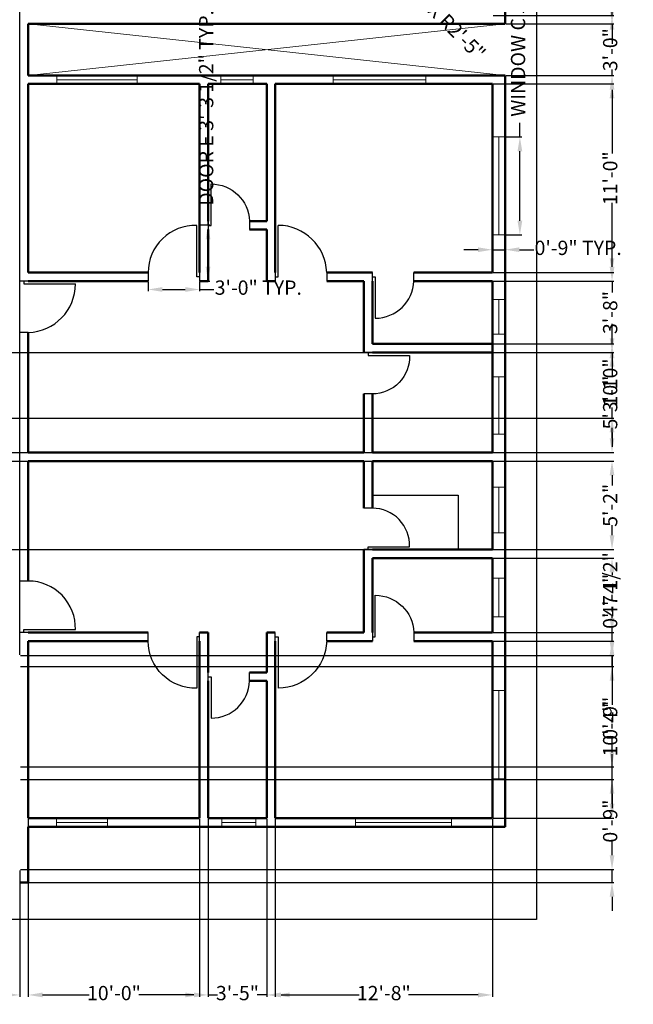
# Model space of a CAD drawing. Units: inches. Extents: x 3237 to 4201, y 2949 to 4053.
# Tile 3 of 5: x 3772 to 4201, y 2949 to 3638. Entities that reach past the tile are written whole.
import ezdxf

# ---------------------------------------------------------------- set-up
doc = ezdxf.new("R2010")
doc.units = ezdxf.units.IN
for name, color, linetype, lineweight in [('A-ANNO-DIMS', 2, 'Continuous', 18), ('A-DOOR', 3, 'Continuous', 25), ('A-FLOR-CASE', 8, 'Continuous', 25), ('A-FLOR-OPEN', 8, 'Continuous', 13), ('A-GLAZ', 4, 'Continuous', 18), ('A-WALL', 7, 'Continuous', 50), ('C-PROP', 6, 'Continuous', 25)]:
    doc.layers.add(name, color=color, linetype=linetype, lineweight=lineweight)
doc.styles.get("Standard").update_dxf_attribs({"font": 'arial.ttf'})
doc.dimstyles.new('ISO-25', dxfattribs={"dimtxt": 10, "dimasz": 10, "dimexe": 1.25, "dimexo": 0.625, "dimtad": 0, "dimdec": 0, "dimlunit": 3, "dimtxsty": 'Standard', "dimcen": 2.5, "dimadec": 0, "dimazin": 0, "dimtfac": 1, "dimtdec": 0, "dimtmove": 0, "dimatfit": 3, "dimfxl": 1, "dimarcsym": 0})

# ---------------------------------------------------------------- blocks, each defined once
blk = doc.blocks.new('DOOR-29-OFFSET-A')
for p, q in [((0, 26), (0, 32)), ((0, 29), (2, 29)), ((2, 29), (2, 0)), ((29, 26), (29, 32))]:
    blk.add_line(p, q)
blk.add_arc((2, 27.02), 27.02, 270, 357.83815)
blk = doc.blocks.new('DOOR-36-OFFSET-A')
for p, q in [((2, 3), (2, 39)), ((0, 6), (0, 0)), ((0, 3), (2, 3)), ((36, 6), (36, 0))]:
    blk.add_line(p, q)
blk.add_arc((2, 4.98), 34.02, 1.71019, 90)
blk = doc.blocks.new('DOOR-29-OFFSET-B')
for p, q in [((27, 3), (27, 32)), ((0, 6), (0, 0)), ((29, 3), (27, 3)), ((29, 6), (29, 0))]:
    blk.add_line(p, q)
blk.add_arc((26.02, 6), 26.02, 87.83815, 180)
blk = doc.blocks.new('DOOR-36-OFFSET-B')
for p, q in [((34, 3), (34, 39)), ((0, 6), (0, 0)), ((36, 3), (34, 3)), ((36, 6), (36, 0))]:
    blk.add_line(p, q)
blk.add_arc((33.01, 6), 33.01, 88.28981, 180)
blk = doc.blocks.new('WIN-61p86IN')
for p, q in [((0, 61.86), (9, 61.86)), ((4.5, 0), (4.5, 61.86)), ((0, 0), (9, 0))]:
    blk.add_line(p, q)
blk = doc.blocks.new('WIN-68p61IN')
for p, q in [((0, 68.61), (9, 68.61)), ((4.5, 0), (4.5, 68.61)), ((0, 0), (9, 0))]:
    blk.add_line(p, q)
blk = doc.blocks.new('COUNTER-L-60x38')
for p, q in [((60, 38), (0, 38)), ((0, 38), (0, 0))]:
    blk.add_line(p, q)
blk = doc.blocks.new('*D23')
at = {"layer": 'A-ANNO-DIMS', "color": 0, "lineweight": -2, "transparency": 16777216}
for p, q in [((3903.41, 3494.25), (3903.41, 3504.25)), ((3898.15, 3494.25), (3904.66, 3494.25)), ((3903.41, 3464.98), (3903.41, 3484.25)), ((3898.15, 3454.98), (3904.66, 3454.98))]:
    blk.add_line(p, q, dxfattribs=at)
at = {"layer": 'A-ANNO-DIMS', "color": 0, "transparency": 16777216}
for points in [[(3901.75, 3484.25), (3905.08, 3484.25), (3903.41, 3494.25)], [(3901.75, 3464.98), (3905.08, 3464.98), (3903.41, 3454.98)]]:
    blk.add_solid(points, dxfattribs=at)
at = {"layer": 'Defpoints', "color": 0, "transparency": 16777216}
for p in [(3897.52, 3494.25), (3903.41, 3494.25), (3897.52, 3454.98)]:
    blk.add_point(p, dxfattribs=at)
at = {"layer": 'A-ANNO-DIMS', "color": 0, "transparency": 16777216, "insert": (3903.41, 3576.25), "char_height": 10, "attachment_point": 5, "rotation": 90}
blk.add_mtext('DOOR E 3\'-3 1/2" TYP.', dxfattribs=at)
blk = doc.blocks.new('*D24')
at = {"layer": 'A-ANNO-DIMS', "color": 0, "lineweight": -2, "transparency": 16777216}
for p, q in [((3861.52, 3454.35), (3861.52, 3447.84)), ((3897.52, 3454.35), (3897.52, 3447.84)), ((3871.52, 3449.09), (3887.52, 3449.09)), ((3897.52, 3449.09), (3907.52, 3449.09))]:
    blk.add_line(p, q, dxfattribs=at)
at = {"layer": 'A-ANNO-DIMS', "color": 0, "transparency": 16777216}
for points in [[(3871.52, 3450.76), (3871.52, 3447.42), (3861.52, 3449.09)], [(3887.52, 3450.76), (3887.52, 3447.42), (3897.52, 3449.09)]]:
    blk.add_solid(points, dxfattribs=at)
at = {"layer": 'Defpoints', "color": 0, "transparency": 16777216}
for p in [(3861.52, 3454.98), (3897.52, 3454.98), (3897.52, 3449.09)]:
    blk.add_point(p, dxfattribs=at)
at = {"layer": 'A-ANNO-DIMS', "color": 0, "transparency": 16777216, "insert": (3938.62, 3449.09), "char_height": 10, "attachment_point": 5}
blk.add_mtext('3\'-0" TYP.', dxfattribs=at)
blk = doc.blocks.new('*D31')
at = {"layer": 'A-ANNO-DIMS', "color": 0, "lineweight": -2, "transparency": 16777216}
for p, q in [((4121.81, 3555.85), (4121.81, 3565.85)), ((4112.15, 3555.85), (4123.06, 3555.85)), ((4121.81, 3497.24), (4121.81, 3545.85)), ((4112.15, 3487.24), (4123.06, 3487.24))]:
    blk.add_line(p, q, dxfattribs=at)
at = {"layer": 'A-ANNO-DIMS', "color": 0, "transparency": 16777216}
for points in [[(4120.15, 3545.85), (4123.48, 3545.85), (4121.81, 3555.85)], [(4120.15, 3497.24), (4123.48, 3497.24), (4121.81, 3487.24)]]:
    blk.add_solid(points, dxfattribs=at)
at = {"layer": 'Defpoints', "color": 0, "transparency": 16777216}
for p in [(4111.52, 3555.85), (4121.81, 3555.85), (4111.52, 3487.24)]:
    blk.add_point(p, dxfattribs=at)
at = {"layer": 'A-ANNO-DIMS', "color": 0, "transparency": 16777216, "insert": (4121.81, 3648.38), "char_height": 10, "attachment_point": 5, "rotation": 90}
blk.add_mtext('WINDOW C 5\'-8 1/2" TYP.', dxfattribs=at)
blk = doc.blocks.new('*D32')
at = {"layer": 'A-ANNO-DIMS', "color": 0, "lineweight": -2, "transparency": 16777216}
for p, q in [((4102.52, 3486.61), (4102.52, 3475.69)), ((4111.52, 3486.61), (4111.52, 3475.69)), ((4092.52, 3476.94), (4082.52, 3476.94)), ((4102.52, 3476.94), (4111.52, 3476.94)), ((4121.52, 3476.94), (4131.52, 3476.94))]:
    blk.add_line(p, q, dxfattribs=at)
at = {"layer": 'A-ANNO-DIMS', "color": 0, "transparency": 16777216}
for points in [[(4092.52, 3478.61), (4092.52, 3475.28), (4102.52, 3476.94)], [(4121.52, 3478.61), (4121.52, 3475.28), (4111.52, 3476.94)]]:
    blk.add_solid(points, dxfattribs=at)
at = {"layer": 'Defpoints', "color": 0, "transparency": 16777216}
for p in [(4102.52, 3487.24), (4111.52, 3487.24), (4111.52, 3476.94)]:
    blk.add_point(p, dxfattribs=at)
at = {"layer": 'A-ANNO-DIMS', "color": 0, "transparency": 16777216, "insert": (4162.62, 3476.94), "char_height": 10, "attachment_point": 5}
blk.add_mtext('0\'-9" TYP.', dxfattribs=at)
blk = doc.blocks.new('*D56')
at = {"layer": 'A-ANNO-DIMS', "color": 0, "lineweight": -2, "transparency": 16777216}
for p, q in [((3777.52, 3078.35), (3777.52, 2953.93)), ((3897.52, 3078.35), (3897.52, 2953.93)), ((3787.52, 2955.18), (3820.19, 2955.18)), ((3887.52, 2955.18), (3854.85, 2955.18))]:
    blk.add_line(p, q, dxfattribs=at)
at = {"layer": 'A-ANNO-DIMS', "color": 0, "transparency": 16777216}
for points in [[(3787.52, 2956.85), (3787.52, 2953.51), (3777.52, 2955.18)], [(3887.52, 2956.85), (3887.52, 2953.51), (3897.52, 2955.18)]]:
    blk.add_solid(points, dxfattribs=at)
at = {"layer": 'Defpoints', "color": 0, "transparency": 16777216}
for p in [(3777.52, 3078.98), (3897.52, 3078.98), (3897.52, 2955.18)]:
    blk.add_point(p, dxfattribs=at)
at = {"layer": 'A-ANNO-DIMS', "color": 0, "transparency": 16777216, "insert": (3837.52, 2955.18), "char_height": 10, "attachment_point": 5}
blk.add_mtext('10\'-0"', dxfattribs=at)
blk = doc.blocks.new('*D57')
at = {"layer": 'A-ANNO-DIMS', "color": 0, "lineweight": -2, "transparency": 16777216}
for p, q in [((3903.52, 3078.35), (3903.52, 2953.93)), ((3944.52, 3078.35), (3944.52, 2953.93)), ((3893.52, 2955.18), (3883.52, 2955.18)), ((3903.52, 2955.18), (3910.11, 2955.18)), ((3944.52, 2955.18), (3937.93, 2955.18)), ((3954.52, 2955.18), (3964.52, 2955.18))]:
    blk.add_line(p, q, dxfattribs=at)
at = {"layer": 'A-ANNO-DIMS', "color": 0, "transparency": 16777216}
for points in [[(3893.52, 2956.85), (3893.52, 2953.51), (3903.52, 2955.18)], [(3954.52, 2956.85), (3954.52, 2953.51), (3944.52, 2955.18)]]:
    blk.add_solid(points, dxfattribs=at)
at = {"layer": 'Defpoints', "color": 0, "transparency": 16777216}
for p in [(3903.52, 3078.98), (3944.52, 3078.98), (3944.52, 2955.18)]:
    blk.add_point(p, dxfattribs=at)
at = {"layer": 'A-ANNO-DIMS', "color": 0, "transparency": 16777216, "insert": (3924.02, 2955.18), "char_height": 10, "attachment_point": 5}
blk.add_mtext('3\'-5"', dxfattribs=at)
blk = doc.blocks.new('*D58')
at = {"layer": 'A-ANNO-DIMS', "color": 0, "lineweight": -2, "transparency": 16777216}
for p, q in [((3950.52, 3078.35), (3950.52, 2953.93)), ((4102.52, 3078.35), (4102.52, 2953.93)), ((3960.52, 2955.18), (4009.19, 2955.18)), ((4092.52, 2955.18), (4043.85, 2955.18))]:
    blk.add_line(p, q, dxfattribs=at)
at = {"layer": 'A-ANNO-DIMS', "color": 0, "transparency": 16777216}
for points in [[(3960.52, 2956.85), (3960.52, 2953.51), (3950.52, 2955.18)], [(4092.52, 2956.85), (4092.52, 2953.51), (4102.52, 2955.18)]]:
    blk.add_solid(points, dxfattribs=at)
at = {"layer": 'Defpoints', "color": 0, "transparency": 16777216}
for p in [(3950.52, 3078.98), (4102.52, 3078.98), (4102.52, 2955.18)]:
    blk.add_point(p, dxfattribs=at)
at = {"layer": 'A-ANNO-DIMS', "color": 0, "transparency": 16777216, "insert": (4026.52, 2955.18), "char_height": 10, "attachment_point": 5}
blk.add_mtext('12\'-8"', dxfattribs=at)
blk = doc.blocks.new('*D61')
at = {"layer": 'A-ANNO-DIMS', "color": 0, "lineweight": -2, "transparency": 16777216}
for p, q in [((3437.15, 3328.98), (4187.57, 3328.98)), ((4186.32, 3318.98), (4186.32, 3311.9)), ((4186.32, 3276.98), (4186.32, 3284.06)), ((3437.15, 3266.98), (4187.57, 3266.98))]:
    blk.add_line(p, q, dxfattribs=at)
at = {"layer": 'A-ANNO-DIMS', "color": 0, "transparency": 16777216}
for points in [[(4184.66, 3318.98), (4187.99, 3318.98), (4186.32, 3328.98)], [(4184.66, 3276.98), (4187.99, 3276.98), (4186.32, 3266.98)]]:
    blk.add_solid(points, dxfattribs=at)
at = {"layer": 'Defpoints', "color": 0, "transparency": 16777216}
for p in [(3436.52, 3328.98), (4186.32, 3328.98), (3436.52, 3266.98)]:
    blk.add_point(p, dxfattribs=at)
at = {"layer": 'A-ANNO-DIMS', "color": 0, "transparency": 16777216, "insert": (4186.32, 3297.98), "char_height": 10, "attachment_point": 5, "rotation": 90}
blk.add_mtext('5\'-2"', dxfattribs=at)
blk = doc.blocks.new('*D62')
at = {"layer": 'A-ANNO-DIMS', "color": 0, "lineweight": -2, "transparency": 16777216}
for p, q in [((3437.15, 3404.98), (4187.57, 3404.98)), ((4186.32, 3394.98), (4186.32, 3387.78)), ((4186.32, 3344.98), (4186.32, 3352.18)), ((3437.15, 3334.98), (4187.57, 3334.98))]:
    blk.add_line(p, q, dxfattribs=at)
at = {"layer": 'A-ANNO-DIMS', "color": 0, "transparency": 16777216}
for points in [[(4184.66, 3394.98), (4187.99, 3394.98), (4186.32, 3404.98)], [(4184.66, 3344.98), (4187.99, 3344.98), (4186.32, 3334.98)]]:
    blk.add_solid(points, dxfattribs=at)
at = {"layer": 'Defpoints', "color": 0, "transparency": 16777216}
for p in [(3436.52, 3404.98), (4186.32, 3404.98), (3436.52, 3334.98)]:
    blk.add_point(p, dxfattribs=at)
at = {"layer": 'A-ANNO-DIMS', "color": 0, "transparency": 16777216, "insert": (4186.32, 3369.98), "char_height": 10, "attachment_point": 5, "rotation": 90}
blk.add_mtext('5\'-10"', dxfattribs=at)
blk = doc.blocks.new('*D63')
at = {"layer": 'A-ANNO-DIMS', "color": 0, "lineweight": -2, "transparency": 16777216}
for p, q in [((4186.32, 3464.98), (4186.32, 3474.98)), ((4103.15, 3454.98), (4187.57, 3454.98)), ((4186.32, 3454.98), (4186.32, 3446.89)), ((4186.32, 3410.98), (4186.32, 3419.07)), ((4103.15, 3410.98), (4187.57, 3410.98)), ((4186.32, 3400.98), (4186.32, 3390.98))]:
    blk.add_line(p, q, dxfattribs=at)
at = {"layer": 'A-ANNO-DIMS', "color": 0, "transparency": 16777216}
for points in [[(4184.66, 3464.98), (4187.99, 3464.98), (4186.32, 3454.98)], [(4184.66, 3400.98), (4187.99, 3400.98), (4186.32, 3410.98)]]:
    blk.add_solid(points, dxfattribs=at)
at = {"layer": 'Defpoints', "color": 0, "transparency": 16777216}
for p in [(4102.52, 3454.98), (4186.32, 3454.98), (4102.52, 3410.98)]:
    blk.add_point(p, dxfattribs=at)
at = {"layer": 'A-ANNO-DIMS', "color": 0, "transparency": 16777216, "insert": (4186.32, 3432.98), "char_height": 10, "attachment_point": 5, "rotation": 90}
blk.add_mtext('3\'-8"', dxfattribs=at)
blk = doc.blocks.new('*D64')
at = {"layer": 'A-ANNO-DIMS', "color": 0, "lineweight": -2, "transparency": 16777216}
for p, q in [((4103.15, 3592.98), (4187.57, 3592.98)), ((4186.32, 3582.98), (4186.32, 3544.31)), ((4186.32, 3470.98), (4186.32, 3509.65)), ((4103.15, 3460.98), (4187.57, 3460.98))]:
    blk.add_line(p, q, dxfattribs=at)
at = {"layer": 'A-ANNO-DIMS', "color": 0, "transparency": 16777216}
for points in [[(4184.66, 3582.98), (4187.99, 3582.98), (4186.32, 3592.98)], [(4184.66, 3470.98), (4187.99, 3470.98), (4186.32, 3460.98)]]:
    blk.add_solid(points, dxfattribs=at)
at = {"layer": 'Defpoints', "color": 0, "transparency": 16777216}
for p in [(4102.52, 3592.98), (4186.32, 3592.98), (4102.52, 3460.98)]:
    blk.add_point(p, dxfattribs=at)
at = {"layer": 'A-ANNO-DIMS', "color": 0, "transparency": 16777216, "insert": (4186.32, 3526.98), "char_height": 10, "attachment_point": 5, "rotation": 90}
blk.add_mtext('11\'-0"', dxfattribs=at)
blk = doc.blocks.new('*D65')
at = {"layer": 'A-ANNO-DIMS', "color": 0, "lineweight": -2, "transparency": 16777216}
for p, q in [((4186.32, 3644.98), (4186.32, 3654.98)), ((4112.15, 3634.98), (4187.57, 3634.98)), ((4186.32, 3634.98), (4186.32, 3630.89)), ((4112.15, 3598.98), (4187.57, 3598.98)), ((4186.32, 3598.98), (4186.32, 3603.07)), ((4186.32, 3588.98), (4186.32, 3578.98))]:
    blk.add_line(p, q, dxfattribs=at)
at = {"layer": 'A-ANNO-DIMS', "color": 0, "transparency": 16777216}
for points in [[(4184.66, 3644.98), (4187.99, 3644.98), (4186.32, 3634.98)], [(4184.66, 3588.98), (4187.99, 3588.98), (4186.32, 3598.98)]]:
    blk.add_solid(points, dxfattribs=at)
at = {"layer": 'Defpoints', "color": 0, "transparency": 16777216}
for p in [(4111.52, 3634.98), (4186.32, 3634.98), (4111.52, 3598.98)]:
    blk.add_point(p, dxfattribs=at)
at = {"layer": 'A-ANNO-DIMS', "color": 0, "transparency": 16777216, "insert": (4186.32, 3616.98), "char_height": 10, "attachment_point": 5, "rotation": 90}
blk.add_mtext('3\'-0"', dxfattribs=at)
blk = doc.blocks.new('*D66')
at = {"layer": 'A-ANNO-DIMS', "color": 0, "lineweight": -2, "transparency": 16777216}
for p, q in [((4186.32, 3698.98), (4186.32, 3708.98)), ((4103.15, 3688.98), (4187.57, 3688.98)), ((4186.32, 3688.98), (4186.32, 3679.1)), ((4186.32, 3640.98), (4186.32, 3650.86)), ((4103.15, 3640.98), (4187.57, 3640.98)), ((4186.32, 3630.98), (4186.32, 3620.98))]:
    blk.add_line(p, q, dxfattribs=at)
at = {"layer": 'A-ANNO-DIMS', "color": 0, "transparency": 16777216}
for points in [[(4184.66, 3698.98), (4187.99, 3698.98), (4186.32, 3688.98)], [(4184.66, 3630.98), (4187.99, 3630.98), (4186.32, 3640.98)]]:
    blk.add_solid(points, dxfattribs=at)
at = {"layer": 'Defpoints', "color": 0, "transparency": 16777216}
for p in [(4102.52, 3688.98), (4186.32, 3688.98), (4102.52, 3640.98)]:
    blk.add_point(p, dxfattribs=at)
at = {"layer": 'A-ANNO-DIMS', "color": 0, "transparency": 16777216, "insert": (4186.32, 3664.98), "char_height": 10, "attachment_point": 5, "rotation": 90}
blk.add_mtext('4\'-0"', dxfattribs=at)
blk = doc.blocks.new('*D70')
at = {"layer": 'A-ANNO-DIMS', "color": 0, "lineweight": -2, "transparency": 16777216}
for p, q in [((4103.15, 3202.98), (4187.57, 3202.98)), ((4186.32, 3192.98), (4186.32, 3158.31)), ((4186.32, 3088.98), (4186.32, 3123.65)), ((4103.15, 3078.98), (4187.57, 3078.98))]:
    blk.add_line(p, q, dxfattribs=at)
at = {"layer": 'A-ANNO-DIMS', "color": 0, "transparency": 16777216}
for points in [[(4184.66, 3192.98), (4187.99, 3192.98), (4186.32, 3202.98)], [(4184.66, 3088.98), (4187.99, 3088.98), (4186.32, 3078.98)]]:
    blk.add_solid(points, dxfattribs=at)
at = {"layer": 'Defpoints', "color": 0, "transparency": 16777216}
for p in [(4102.52, 3202.98), (4186.32, 3202.98), (4102.52, 3078.98)]:
    blk.add_point(p, dxfattribs=at)
at = {"layer": 'A-ANNO-DIMS', "color": 0, "transparency": 16777216, "insert": (4186.32, 3140.98), "char_height": 10, "attachment_point": 5, "rotation": 90}
blk.add_mtext('10\'-4"', dxfattribs=at)
blk = doc.blocks.new('*D71')
at = {"layer": 'A-ANNO-DIMS', "color": 0, "lineweight": -2, "transparency": 16777216}
for p, q in [((4103.15, 3260.98), (4187.57, 3260.98)), ((4186.32, 3250.98), (4186.32, 3249.1)), ((4186.32, 3218.98), (4186.32, 3220.86)), ((4103.15, 3208.98), (4187.57, 3208.98))]:
    blk.add_line(p, q, dxfattribs=at)
at = {"layer": 'A-ANNO-DIMS', "color": 0, "transparency": 16777216}
for points in [[(4184.66, 3250.98), (4187.99, 3250.98), (4186.32, 3260.98)], [(4184.66, 3218.98), (4187.99, 3218.98), (4186.32, 3208.98)]]:
    blk.add_solid(points, dxfattribs=at)
at = {"layer": 'Defpoints', "color": 0, "transparency": 16777216}
for p in [(4102.52, 3260.98), (4186.32, 3260.98), (4102.52, 3208.98)]:
    blk.add_point(p, dxfattribs=at)
at = {"layer": 'A-ANNO-DIMS', "color": 0, "transparency": 16777216, "insert": (4186.32, 3234.98), "char_height": 10, "attachment_point": 5, "rotation": 90}
blk.add_mtext('4\'-4"', dxfattribs=at)
blk = doc.blocks.new('*D74')
at = {"layer": 'A-ANNO-DIMS', "color": 0, "lineweight": -2, "transparency": 16777216}
for p, q in [((4186.32, 3414.98), (4186.32, 3424.98)), ((3377.15, 3404.98), (4187.57, 3404.98)), ((4186.32, 3404.98), (4186.32, 3399.78)), ((4186.32, 3358.98), (4186.32, 3364.18)), ((3377.15, 3358.98), (4187.57, 3358.98)), ((4186.32, 3348.98), (4186.32, 3338.98))]:
    blk.add_line(p, q, dxfattribs=at)
at = {"layer": 'A-ANNO-DIMS', "color": 0, "transparency": 16777216}
for points in [[(4184.66, 3414.98), (4187.99, 3414.98), (4186.32, 3404.98)], [(4184.66, 3348.98), (4187.99, 3348.98), (4186.32, 3358.98)]]:
    blk.add_solid(points, dxfattribs=at)
at = {"layer": 'Defpoints', "color": 0, "transparency": 16777216}
for p in [(3376.52, 3404.98), (4186.32, 3404.98), (3376.52, 3358.98)]:
    blk.add_point(p, dxfattribs=at)
at = {"layer": 'A-ANNO-DIMS', "color": 0, "transparency": 16777216, "insert": (4186.32, 3381.98), "char_height": 10, "attachment_point": 5, "rotation": 90}
blk.add_mtext('3\'-10"', dxfattribs=at)
blk = doc.blocks.new('*D80')
at = {"layer": 'A-ANNO-DIMS', "color": 0, "lineweight": -2, "transparency": 16777216}
for p, q in [((3675.52, 3042.35), (3675.52, 2953.93)), ((3771.52, 3042.35), (3771.52, 2953.93)), ((3685.52, 2955.18), (3709.6, 2955.18)), ((3761.52, 2955.18), (3737.44, 2955.18))]:
    blk.add_line(p, q, dxfattribs=at)
at = {"layer": 'A-ANNO-DIMS', "color": 0, "transparency": 16777216}
for points in [[(3685.52, 2956.85), (3685.52, 2953.51), (3675.52, 2955.18)], [(3761.52, 2956.85), (3761.52, 2953.51), (3771.52, 2955.18)]]:
    blk.add_solid(points, dxfattribs=at)
at = {"layer": 'Defpoints', "color": 0, "transparency": 16777216}
for p in [(3675.52, 3042.98), (3771.52, 3042.98), (3771.52, 2955.18)]:
    blk.add_point(p, dxfattribs=at)
at = {"layer": 'A-ANNO-DIMS', "color": 0, "transparency": 16777216, "insert": (3723.52, 2955.18), "char_height": 10, "attachment_point": 5}
blk.add_mtext('8\'-0"', dxfattribs=at)
blk = doc.blocks.new('*D83')
at = {"layer": 'A-ANNO-DIMS', "color": 0, "lineweight": -2, "transparency": 16777216}
for p, q in [((3713.52, 3960.78), (3703.52, 3960.78)), ((3723.52, 3193.4), (3723.52, 3962.03)), ((3723.52, 3960.78), (3733.4, 3960.78)), ((3771.52, 3960.78), (3761.64, 3960.78)), ((3771.52, 3193.4), (3771.52, 3962.03)), ((3781.52, 3960.78), (3791.52, 3960.78))]:
    blk.add_line(p, q, dxfattribs=at)
at = {"layer": 'A-ANNO-DIMS', "color": 0, "transparency": 16777216}
for points in [[(3713.52, 3962.45), (3713.52, 3959.11), (3723.52, 3960.78)], [(3781.52, 3962.45), (3781.52, 3959.11), (3771.52, 3960.78)]]:
    blk.add_solid(points, dxfattribs=at)
at = {"layer": 'Defpoints', "color": 0, "transparency": 16777216}
for p in [(3771.52, 3960.78), (3723.52, 3192.78), (3771.52, 3192.78)]:
    blk.add_point(p, dxfattribs=at)
at = {"layer": 'A-ANNO-DIMS', "color": 0, "transparency": 16777216, "insert": (3747.52, 3960.78), "char_height": 10, "attachment_point": 5}
blk.add_mtext('4\'-0"', dxfattribs=at)
blk = doc.blocks.new('*D84')
at = {"layer": 'A-ANNO-DIMS', "color": 0, "lineweight": -2, "transparency": 16777216}
for p, q in [((4186.32, 3124.98), (4186.32, 3134.98)), ((3772.15, 3114.98), (4187.57, 3114.98)), ((4186.32, 3105.98), (4186.32, 3114.98)), ((3772.15, 3105.98), (4187.57, 3105.98)), ((4186.32, 3095.98), (4186.32, 3085.98))]:
    blk.add_line(p, q, dxfattribs=at)
at = {"layer": 'A-ANNO-DIMS', "color": 0, "transparency": 16777216}
for points in [[(4184.66, 3124.98), (4187.99, 3124.98), (4186.32, 3114.98)], [(4184.66, 3095.98), (4187.99, 3095.98), (4186.32, 3105.98)]]:
    blk.add_solid(points, dxfattribs=at)
at = {"layer": 'Defpoints', "color": 0, "transparency": 16777216}
for p in [(3771.52, 3114.98), (4186.32, 3114.98), (3771.52, 3105.98)]:
    blk.add_point(p, dxfattribs=at)
at = {"layer": 'A-ANNO-DIMS', "color": 0, "transparency": 16777216, "insert": (4186.32, 3148.9), "char_height": 10, "attachment_point": 5, "rotation": 90}
blk.add_mtext('0\'-9"', dxfattribs=at)
blk = doc.blocks.new('*D85')
at = {"layer": 'A-ANNO-DIMS', "color": 0, "lineweight": -2, "transparency": 16777216}
for p, q in [((4186.32, 3202.78), (4186.32, 3212.78)), ((3772.15, 3192.78), (4187.57, 3192.78)), ((4186.32, 3185.23), (4186.32, 3192.78)), ((3772.15, 3185.23), (4187.57, 3185.23)), ((4186.32, 3175.23), (4186.32, 3165.23))]:
    blk.add_line(p, q, dxfattribs=at)
at = {"layer": 'A-ANNO-DIMS', "color": 0, "transparency": 16777216}
for points in [[(4184.66, 3202.78), (4187.99, 3202.78), (4186.32, 3192.78)], [(4184.66, 3175.23), (4187.99, 3175.23), (4186.32, 3185.23)]]:
    blk.add_solid(points, dxfattribs=at)
at = {"layer": 'Defpoints', "color": 0, "transparency": 16777216}
for p in [(3771.52, 3192.78), (4186.32, 3192.78), (3771.52, 3185.23)]:
    blk.add_point(p, dxfattribs=at)
at = {"layer": 'A-ANNO-DIMS', "color": 0, "transparency": 16777216, "insert": (4186.32, 3238.34), "char_height": 10, "attachment_point": 5, "rotation": 90}
blk.add_mtext('0\'-7 1/2"', dxfattribs=at)
blk = doc.blocks.new('*D87')
at = {"layer": 'A-ANNO-DIMS', "color": 0, "lineweight": -2, "transparency": 16777216}
for p, q in [((4186.32, 3052.98), (4186.32, 3062.98)), ((3772.15, 3042.98), (4187.57, 3042.98)), ((4186.32, 3033.98), (4186.32, 3042.98)), ((3778, 3033.98), (4187.57, 3033.98)), ((4186.32, 3023.98), (4186.32, 3013.98))]:
    blk.add_line(p, q, dxfattribs=at)
at = {"layer": 'A-ANNO-DIMS', "color": 0, "transparency": 16777216}
for points in [[(4184.66, 3052.98), (4187.99, 3052.98), (4186.32, 3042.98)], [(4184.66, 3023.98), (4187.99, 3023.98), (4186.32, 3033.98)]]:
    blk.add_solid(points, dxfattribs=at)
at = {"layer": 'Defpoints', "color": 0, "transparency": 16777216}
for p in [(3771.52, 3042.98), (4186.32, 3042.98), (3777.38, 3033.98)]:
    blk.add_point(p, dxfattribs=at)
at = {"layer": 'A-ANNO-DIMS', "color": 0, "transparency": 16777216, "insert": (4186.32, 3076.9), "char_height": 10, "attachment_point": 5, "rotation": 90}
blk.add_mtext('0\'-9"', dxfattribs=at)
blk = doc.blocks.new('*D93')
at = {"layer": 'A-ANNO-DIMS', "color": 0, "lineweight": -2, "transparency": 16777216}
for p, q in [((4018.52, 3686.98), (4039.03, 3666.47)), ((4053.17, 3652.33), (4046.1, 3659.4))]:
    blk.add_line(p, q, dxfattribs=at)
at = {"layer": 'A-ANNO-DIMS', "color": 0, "transparency": 16777216}
blk.add_solid([(4047.28, 3660.58), (4044.92, 3658.22), (4039.03, 3666.47)], dxfattribs=at)
at = {"layer": 'Defpoints', "color": 0, "transparency": 16777216}
for p in [(4018.52, 3686.98), (4039.03, 3666.47)]:
    blk.add_point(p, dxfattribs=at)
at = {"layer": 'A-ANNO-DIMS', "color": 0, "transparency": 16777216, "insert": (4074.05, 3631.45), "char_height": 10, "attachment_point": 5, "rotation": 314.99953}
blk.add_mtext('2X R2\'-5"', dxfattribs=at)

msp = doc.modelspace()

# ---------------------------------------------------------------- linework, layer by layer
at = {"layer": 'A-FLOR-OPEN'}
for p, q in [((3777.52, 3598.98), (4111.52, 3634.98)), ((4111.52, 3598.98), (3777.52, 3634.98))]:
    msp.add_line(p, q, dxfattribs=at)
at = {"layer": 'A-GLAZ'}
for p, q in [((3797.53, 3598.98), (3797.53, 3592.98)), ((3853.71, 3598.98), (3853.71, 3592.98)), ((3912.44, 3592.98), (3912.44, 3598.98)), ((3934.97, 3592.98), (3934.97, 3598.98)), ((3991.04, 3592.98), (3991.04, 3598.98)), ((4055.93, 3592.98), (4055.93, 3598.98)), ((3853.71, 3595.98), (3797.53, 3595.98)), ((3934.97, 3595.98), (3912.44, 3595.98)), ((4055.93, 3595.98), (3991.04, 3595.98)), ((4102.52, 3442.14), (4111.52, 3442.14)), ((4107.02, 3417.7), (4107.02, 3442.14)), ((4102.52, 3417.7), (4111.52, 3417.7)), ((4102.52, 3417.7), (4111.52, 3417.7)), ((4102.52, 3387.9), (4111.52, 3387.9)), ((4107.02, 3347.84), (4107.02, 3387.9)), ((4102.52, 3347.84), (4111.52, 3347.84)), ((4102.52, 3310.79), (4111.52, 3310.79)), ((4107.02, 3278.68), (4107.02, 3310.79)), ((4102.52, 3278.68), (4111.52, 3278.68)), ((4102.52, 3246.88), (4111.52, 3246.88)), ((4107.02, 3219.91), (4107.02, 3246.88)), ((4102.52, 3219.91), (4111.52, 3219.91)), ((3797.38, 3072.98), (3797.38, 3078.98)), ((3797.38, 3078.98), (3797.38, 3075.98)), ((3797.38, 3075.98), (3832.9, 3075.98)), ((3832.9, 3078.98), (3832.9, 3072.98)), ((3912.99, 3078.98), (3912.99, 3072.98)), ((3912.99, 3075.98), (3936.79, 3075.98)), ((3936.79, 3078.98), (3936.79, 3072.98)), ((4006.66, 3078.98), (4006.66, 3072.98)), ((4006.66, 3075.98), (4073.8, 3075.98)), ((4073.8, 3078.98), (4073.8, 3072.98)), ((3832.9, 3072.98), (3797.38, 3072.98))]:
    msp.add_line(p, q, dxfattribs=at)
at = {"layer": 'A-WALL'}
for p, q in [((4111.52, 3634.98), (4111.52, 3885.98)), ((4102.52, 3634.98), (3777.52, 3634.98)), ((3777.52, 3634.98), (3777.52, 3598.98)), ((4102.52, 3634.98), (4111.52, 3634.98)), ((4102.52, 3598.98), (3777.52, 3598.98)), ((4102.52, 3598.98), (4111.52, 3598.98)), ((4111.52, 3072.98), (4111.52, 3598.98)), ((3777.52, 3592.98), (3777.52, 3460.98)), ((3897.52, 3592.98), (3777.52, 3592.98)), ((3897.52, 3592.98), (3897.52, 3460.98)), ((3903.52, 3592.98), (3903.52, 3496.98)), ((3944.52, 3592.98), (3903.52, 3592.98)), ((3944.52, 3592.98), (3944.52, 3496.98)), ((4102.52, 3592.98), (3950.52, 3592.98)), ((3950.52, 3592.98), (3950.52, 3460.98)), ((4102.52, 3460.98), (4102.52, 3592.98)), ((3944.52, 3496.98), (3932.52, 3496.98)), ((3903.52, 3490.98), (3903.52, 3460.98)), ((3944.52, 3490.98), (3932.52, 3490.98)), ((3944.52, 3490.98), (3944.52, 3460.98)), ((3861.52, 3460.98), (3777.52, 3460.98)), ((3903.52, 3460.98), (3903.52, 3454.98)), ((3944.52, 3460.98), (3944.52, 3454.98)), ((4018.52, 3460.98), (3986.52, 3460.98)), ((4102.52, 3460.98), (4047.52, 3460.98)), ((3861.52, 3454.98), (3777.52, 3454.98)), ((3903.52, 3454.98), (3897.52, 3454.98)), ((3950.52, 3454.98), (3944.52, 3454.98)), ((4012.52, 3454.98), (3986.52, 3454.98)), ((4012.52, 3404.98), (4012.52, 3454.98)), ((4018.52, 3410.98), (4018.52, 3454.98)), ((4102.52, 3454.98), (4047.52, 3454.98)), ((4102.52, 3334.98), (4102.52, 3454.98)), ((3777.52, 3418.98), (3777.52, 3334.98)), ((4102.52, 3410.98), (4018.52, 3410.98)), ((4102.52, 3404.98), (4018.52, 3404.98)), ((4012.52, 3334.98), (4012.52, 3375.98)), ((4018.52, 3334.98), (4018.52, 3375.98)), ((4012.52, 3334.98), (3777.52, 3334.98)), ((4102.52, 3334.98), (4018.52, 3334.98)), ((3777.52, 3328.98), (3777.52, 3244.98)), ((4012.52, 3328.98), (3777.52, 3328.98)), ((4012.52, 3295.98), (4012.52, 3328.98)), ((4102.52, 3328.98), (4018.52, 3328.98)), ((4018.52, 3295.98), (4018.52, 3328.98)), ((4102.52, 3266.98), (4102.52, 3328.98)), ((4012.52, 3208.98), (4012.52, 3266.98)), ((4102.52, 3266.98), (4018.52, 3266.98)), ((4102.52, 3260.98), (4018.52, 3260.98)), ((4018.52, 3208.98), (4018.52, 3260.98)), ((4102.52, 3208.98), (4102.52, 3260.98)), ((3861.52, 3208.98), (3777.52, 3208.98)), ((3903.52, 3208.98), (3897.52, 3208.98)), ((3903.52, 3208.98), (3903.52, 3180.98)), ((3950.52, 3208.98), (3944.52, 3208.98)), ((3944.52, 3208.98), (3944.52, 3208.98)), ((3944.52, 3208.98), (3944.52, 3180.98)), ((4012.52, 3208.98), (3986.52, 3208.98)), ((4102.52, 3208.98), (4047.52, 3208.98)), ((3777.52, 3202.98), (3777.52, 3078.98)), ((3861.52, 3202.98), (3777.52, 3202.98)), ((3897.52, 3202.98), (3897.52, 3078.98)), ((3950.52, 3078.98), (3950.52, 3202.98)), ((4018.52, 3202.98), (3986.52, 3202.98)), ((4102.52, 3202.98), (4047.52, 3202.98)), ((4102.52, 3078.98), (4102.52, 3202.98)), ((3944.52, 3180.98), (3932.52, 3180.98)), ((3903.52, 3174.98), (3903.52, 3078.98)), ((3944.52, 3174.98), (3932.52, 3174.98)), ((3944.52, 3174.98), (3944.52, 3078.98)), ((3897.52, 3078.98), (3777.52, 3078.98)), ((3944.52, 3078.98), (3903.52, 3078.98)), ((4102.52, 3078.98), (3950.52, 3078.98)), ((4102.52, 3078.98), (3970.52, 3078.98)), ((4102.52, 3072.98), (3777.38, 3072.98)), ((3777.38, 3033.98), (3777.38, 3072.98)), ((4102.52, 3072.98), (4111.52, 3072.98)), ((3771.38, 3033.98), (3777.38, 3033.98))]:
    msp.add_line(p, q, dxfattribs=at)
at = {"layer": 'C-PROP'}
for p, q in [((4133.52, 3907.98), (4133.52, 3007.98)), ((4133.52, 3007.98), (3353.52, 3007.98))]:
    msp.add_line(p, q, dxfattribs=at)

# ---------------------------------------------------------------- block references
at = {"layer": 'A-DOOR', "extrusion": (0, 0, -1), "zscale": -1}
for name, p, rotation in [('DOOR-29-OFFSET-A', (-3903.52, 3522.98), 180), ('DOOR-29-OFFSET-B', (-4012.52, 3375.98), 89.99999999999496), ('DOOR-29-OFFSET-A', (-4018.52, 3234.98), 180), ('DOOR-36-OFFSET-B', (-3861.52, 3208.98), 180), ('DOOR-36-OFFSET-A', (-3950.52, 3208.98), 180)]:
    msp.add_blockref(name, p, dxfattribs=dict(at, rotation=rotation))
at = {"layer": 'A-DOOR'}
for name, p in [('DOOR-36-OFFSET-B', (3861.52, 3454.98)), ('DOOR-36-OFFSET-A', (3950.52, 3454.98)), ('DOOR-29-OFFSET-A', (4018.52, 3428.98)), ('DOOR-29-OFFSET-A', (3903.52, 3148.98))]:
    msp.add_blockref(name, p, dxfattribs=at)
for name, p, rotation in [('DOOR-36-OFFSET-A', (3771.52, 3454.98), 270.0000000000005), ('DOOR-29-OFFSET-B', (4012.52, 3295.98), 269.9999999999981), ('DOOR-36-OFFSET-B', (3771.52, 3244.98), 269.9999999999984)]:
    msp.add_blockref(name, p, dxfattribs=dict(at, rotation=rotation))
at = {"layer": 'A-FLOR-CASE', "extrusion": (0, 0, -1), "zscale": -1}
msp.add_blockref('COUNTER-L-60x38', (-4078.52, 3266.98), dxfattribs=at)
at = {"layer": 'A-GLAZ'}
for name, p in [('WIN-68p61IN', (4102.52, 3487.24)), ('WIN-61p86IN', (4102.52, 3106.57))]:
    msp.add_blockref(name, p, dxfattribs=at)

# ---------------------------------------------------------------- dimensions: what is measured, and where the dimension line sits
at = {"layer": 'A-ANNO-DIMS'}
for base, p1, p2, picture, middle in [((3771.52, 3960.78), (3723.52, 3192.78), (3771.52, 3192.78), '*D83', (3747.52, 3960.78)), ((3897.52, 2955.18), (3777.52, 3078.98), (3897.52, 3078.98), '*D56', (3837.52, 2955.18)), ((3944.52, 2955.18), (3903.52, 3078.98), (3944.52, 3078.98), '*D57', (3924.02, 2955.18)), ((4102.52, 2955.18), (3950.52, 3078.98), (4102.52, 3078.98), '*D58', (4026.52, 2955.18)), ((3771.52, 2955.18), (3675.52, 3042.98), (3771.52, 3042.98), '*D80', (3723.52, 2955.18))]:
    dim = msp.add_linear_dim(base=base, p1=p1, p2=p2, dimstyle='ISO-25', override={"dimdec": 1, "dimlfac": 1, "dimrnd": 0, "dimzin": 1, "dimdsep": 46, "dimlunit": 4, "dimfrac": 2}, dxfattribs=at)
    dim.commit()
    dim.dimension.update_dxf_attribs({"geometry": picture, "text_midpoint": middle})
for base, p1, p2, text, picture, middle in [((4121.81, 3555.85), (4111.52, 3487.24), (4111.52, 3555.85), 'WINDOW C <> TYP.', '*D31', (4121.81, 3648.38)), ((3903.41, 3494.25), (3897.52, 3454.98), (3897.52, 3494.25), 'DOOR E <> TYP.', '*D23', (3903.41, 3576.25))]:
    dim = msp.add_linear_dim(base=base, p1=p1, p2=p2, angle=90, text=text, dimstyle='ISO-25', override={"dimdec": 1, "dimlfac": 1, "dimrnd": 0, "dimzin": 1, "dimdsep": 46, "dimlunit": 4, "dimfrac": 2}, dxfattribs=at)
    dim.commit()
    dim.dimension.update_dxf_attribs({"geometry": picture, "text_midpoint": middle})
for base, p1, p2, picture, middle in [((4186.32, 3688.98), (4102.52, 3640.98), (4102.52, 3688.98), '*D66', (4186.32, 3664.98)), ((4186.32, 3634.98), (4111.52, 3598.98), (4111.52, 3634.98), '*D65', (4186.32, 3616.98)), ((4186.32, 3592.98), (4102.52, 3460.98), (4102.52, 3592.98), '*D64', (4186.32, 3526.98)), ((4186.32, 3454.98), (4102.52, 3410.98), (4102.52, 3454.98), '*D63', (4186.32, 3432.98)), ((4186.32, 3404.98), (3376.52, 3358.98), (3376.52, 3404.98), '*D74', (4186.32, 3381.98)), ((4186.32, 3404.98), (3436.52, 3334.98), (3436.52, 3404.98), '*D62', (4186.32, 3369.98)), ((4186.32, 3328.98), (3436.52, 3266.98), (3436.52, 3328.98), '*D61', (4186.32, 3297.98)), ((4186.3217, 3192.7764), (3771.5217, 3185.2339), (3771.5217, 3192.7764), '*D85', (4186.3217, 3238.3434)), ((4186.32, 3260.98), (4102.52, 3208.98), (4102.52, 3260.98), '*D71', (4186.32, 3234.98)), ((4186.32, 3202.98), (4102.52, 3078.98), (4102.52, 3202.98), '*D70', (4186.32, 3140.98)), ((4186.32, 3114.98), (3771.52, 3105.98), (3771.52, 3114.98), '*D84', (4186.32, 3148.9)), ((4186.32, 3042.98), (3777.38, 3033.98), (3771.52, 3042.98), '*D87', (4186.32, 3076.9))]:
    dim = msp.add_linear_dim(base=base, p1=p1, p2=p2, angle=90, dimstyle='ISO-25', override={"dimdec": 1, "dimlfac": 1, "dimrnd": 0, "dimzin": 1, "dimdsep": 46, "dimlunit": 4, "dimfrac": 2}, dxfattribs=at)
    dim.commit()
    dim.dimension.update_dxf_attribs({"geometry": picture, "text_midpoint": middle})
dim = msp.add_radius_dim(center=(4018.52, 3686.98), mpoint=(4039.03, 3666.47), text='2X <>', dimstyle='ISO-25', override={"dimdec": 1, "dimlfac": 1, "dimrnd": 0, "dimzin": 1, "dimdsep": 46, "dimlunit": 4, "dimfrac": 2}, dxfattribs=at)
dim.commit()
dim.dimension.update_dxf_attribs({"geometry": '*D93', "text_midpoint": (4074.05, 3631.45)})
for base, p1, p2, picture, middle in [((4111.52, 3476.94), (4102.52, 3487.24), (4111.52, 3487.24), '*D32', (4162.62, 3476.94)), ((3897.52, 3449.09), (3861.52, 3454.98), (3897.52, 3454.98), '*D24', (3938.62, 3449.09))]:
    dim = msp.add_linear_dim(base=base, p1=p1, p2=p2, text='<> TYP.', dimstyle='ISO-25', override={"dimdec": 1, "dimlfac": 1, "dimrnd": 0, "dimzin": 1, "dimdsep": 46, "dimlunit": 4, "dimfrac": 2}, dxfattribs=at)
    dim.commit()
    dim.dimension.update_dxf_attribs({"geometry": picture, "text_midpoint": middle})

doc.saveas('drawing.dxf')
